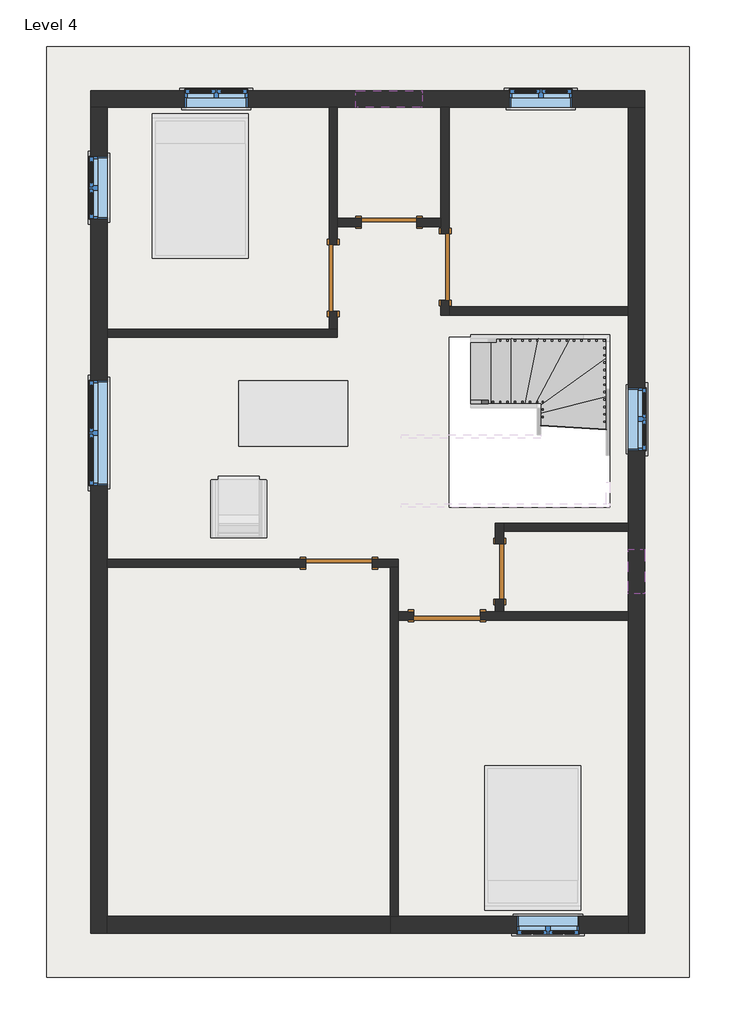
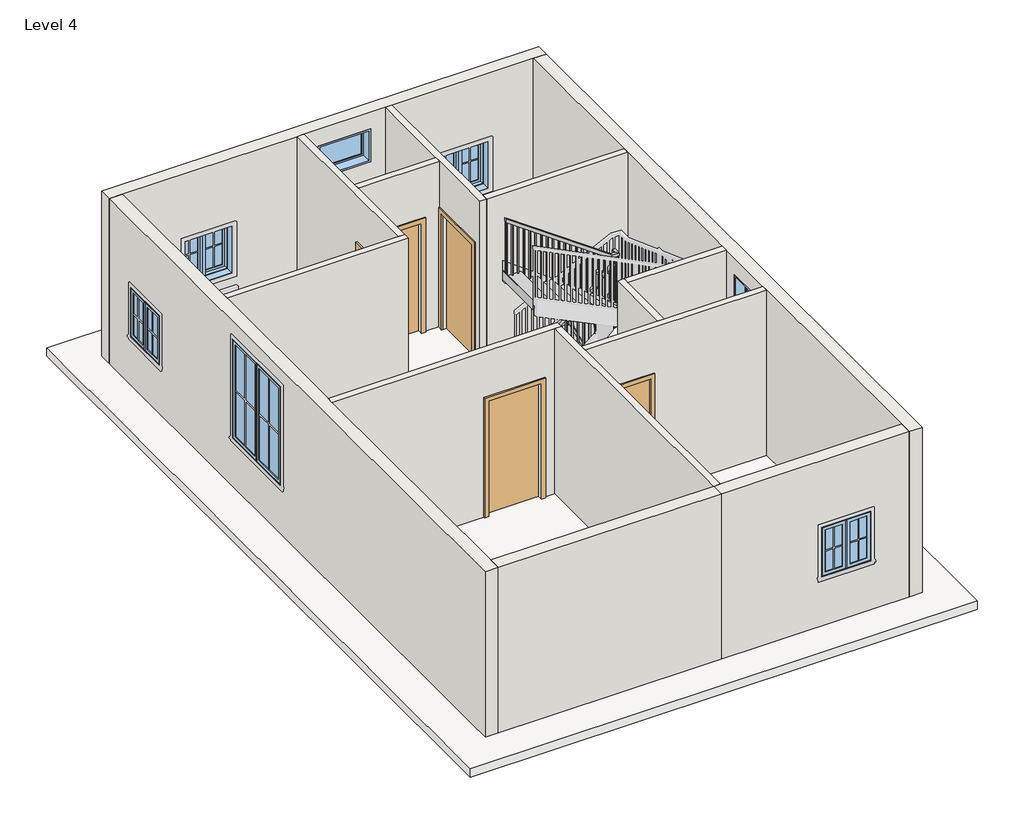
# One storey, part 1 of 2: 15 walls, 8 windows, 6 doors, 1 railing, 1 roof, 1 stair flight.
"""IFC4 building model written with IfcOpenShell, lengths in millimetres."""

from ifc_helpers import new_model, si_unit, frame, origin, place, context, project, spatial, polyline, outline, extrude, faceted_brep, transform, mapped, element, save
from components import door_d8f5dbb5, door_f2b275c1, door_e5f9f3c4, door_305aa2a5, stair_flight_52755f88, window_80340324, window_bb95b1c9, window_339605e1, window_9ac97e1a

model = new_model("IFC4")

# Units and contexts
model_context = context("Model", 3, world=origin())
ifc_project = project(units=[si_unit("LENGTHUNIT", "METRE", prefix="MILLI")], contexts=[model_context])

# Site, building, storey
site = spatial("IfcSite", under=ifc_project)
building = spatial("IfcBuilding", under=site)
storey = spatial("IfcBuildingStorey", under=building, Name="Level 4", Elevation=6400.8)

# Doors
placement = place(None, origin())
door_shape = door_d8f5dbb5(model_context)
element("IfcDoor", 1, ObjectType="Single-Flush : 30\" x 80\"", at=placement, inside=storey, context=model_context, shape_type="MappedRepresentation", body=[
    mapped(door_shape, transform((-963.1415084, 4519.6435985, 6400.8), x_axis=(1.0, 0.0, 0.0), y_axis=(0.0, 1.0, 0.0), z_axis=(0.0, 0.0, 1.0))),
])
door_2_shape = door_f2b275c1(model_context)
element("IfcDoor", 2, ObjectType="Single-Flush : 30\" x 80\"", at=placement, inside=storey, context=model_context, shape_type="MappedRepresentation", body=[
    mapped(door_2_shape, transform((554.5084916, -280.9564015, 6400.8), x_axis=(0.0, 1.0, 0.0), y_axis=(-1.0, 0.0, 0.0), z_axis=(0.0, 0.0, 1.0))),
])
door_3_shape = door_e5f9f3c4(model_context)
element("IfcDoor", 3, ObjectType="Single-Flush : 36\" x 84\"", at=placement, inside=storey, context=model_context, shape_type="MappedRepresentation", body=[
    mapped(door_3_shape, transform((-194.7915084, 3910.0435985, 6400.8), x_axis=(0.0, -1.0, 0.0), y_axis=(1.0, 0.0, 0.0), z_axis=(0.0, 0.0, 1.0))),
])
element("IfcDoor", 4, ObjectType="Single-Flush : 36\" x 84\"", at=placement, inside=storey, context=model_context, shape_type="MappedRepresentation", body=[
    mapped(door_3_shape, transform((-1655.2915084, -166.6564015, 6400.8), x_axis=(1.0, 0.0, 0.0), y_axis=(0.0, 1.0, 0.0), z_axis=(0.0, 0.0, 1.0))),
])
element("IfcDoor", 5, ObjectType="Single-Flush : 36\" x 84\"", at=placement, inside=storey, context=model_context, shape_type="MappedRepresentation", body=[
    mapped(door_3_shape, transform((-169.3915084, -890.5564015, 6400.8), x_axis=(-1.0, 0.0, 0.0), y_axis=(0.0, -1.0, 0.0), z_axis=(0.0, 0.0, 1.0))),
])
door_4_shape = door_305aa2a5(model_context)
element("IfcDoor", 6, ObjectType="Single-Flush : 36\" x 84\"", at=placement, inside=storey, context=model_context, shape_type="MappedRepresentation", body=[
    mapped(door_4_shape, transform((-1731.4915084, 3757.6435985, 6400.8), x_axis=(0.0, -1.0, 0.0), y_axis=(1.0, 0.0, 0.0), z_axis=(0.0, 0.0, 1.0))),
])

# Railing
element("IfcRailing", 7, ObjectType="Handrail - Rectangular", at=placement, inside=storey, context=model_context, shape_type="SolidModel", body=[
    faceted_brep([(158.6923968, 2074.8935985, 7484.5333333), (158.6923968, 2074.8935985, 7420.8053174), (158.6923968, 2024.0935985, 7420.8053174), (158.6923968, 2024.0935985, 7484.5333333), (1047.1901835, 2074.8935985, 8157.532376), (1097.9901835, 2074.8935985, 8132.2831856), (1097.9901835, 2024.0935985, 8132.2831856), (1047.1901835, 2024.0935985, 8157.532376), (1047.1901835, 2074.8935985, 8411.8303182), (1097.9901835, 2074.8935985, 8361.0303182), (1097.9901835, 2024.0935985, 8361.0303182), (1047.1901835, 2024.0935985, 8411.8303182), (1174.1901835, 2074.8935985, 8411.8303182), (1174.1901835, 2074.8935985, 8361.0303182), (1123.3901835, 2024.0935985, 8361.0303182), (1123.3901835, 2024.0935985, 8411.8303182), (1174.1901835, 1947.8935985, 8411.8303182), (1174.1901835, 1922.7437783, 8361.0303182), (1123.3901835, 1922.7437783, 8361.0303182), (1123.3901835, 1947.8935985, 8411.8303182), (1174.1901835, 1627.4476133, 8832.13697), (1174.1901835, 1576.6476133, 8814.9805221), (1123.3901835, 1576.6476133, 8814.9805221), (1123.3901835, 1627.4476133, 8832.13697), (1174.1901835, 1627.4476133, 9053.3821577), (1174.1901835, 1576.6476133, 9002.5821577), (1123.3901835, 1576.6476133, 9002.5821577), (1123.3901835, 1627.4476133, 9053.3821577), (1174.1901835, 1500.4476133, 9053.3821577), (1174.1901835, 1500.4476133, 9002.5821577), (1123.3901835, 1551.2476133, 9002.5821577), (1123.3901835, 1551.2476133, 9053.3821577), (1047.1901835, 1500.4476133, 9053.3821577), (1030.9951821, 1500.4476133, 9002.5821577), (1030.9951821, 1551.2476133, 9002.5821577), (1047.1901835, 1551.2476133, 9053.3821577), (-798.3242294, 1500.4476133, 10363.2), (-798.3242294, 1551.2476133, 10363.2), (-798.3242294, 1551.2476133, 10300.9059138), (-798.3242294, 1500.4476133, 10300.9059138)], [[[0, 1, 2, 3]], [[1, 0, 4, 5]], [[2, 1, 5, 6]], [[3, 2, 6, 7]], [[0, 3, 7, 4]], [[5, 4, 8, 9]], [[6, 5, 9, 10]], [[7, 6, 10, 11]], [[4, 7, 11, 8]], [[9, 8, 12, 13]], [[10, 9, 13, 14]], [[11, 10, 14, 15]], [[8, 11, 15, 12]], [[13, 12, 16, 17]], [[14, 13, 17, 18]], [[15, 14, 18, 19]], [[12, 15, 19, 16]], [[17, 16, 20, 21]], [[18, 17, 21, 22]], [[19, 18, 22, 23]], [[16, 19, 23, 20]], [[21, 20, 24, 25]], [[22, 21, 25, 26]], [[23, 22, 26, 27]], [[20, 23, 27, 24]], [[25, 24, 28, 29]], [[26, 25, 29, 30]], [[27, 26, 30, 31]], [[24, 27, 31, 28]], [[29, 28, 32, 33]], [[30, 29, 33, 34]], [[31, 30, 34, 35]], [[28, 31, 35, 32]], [[36, 37, 38, 39]], [[33, 32, 36, 39]], [[34, 33, 39, 38]], [[35, 34, 38, 37]], [[32, 35, 37, 36]]]),
    extrude(outline(polyline([(10282.2830025, -772.0848165), (10295.8033683, -791.1348165), (9279.4666667, -791.1348165), (9279.4666667, -772.0848165), (10282.2830025, -772.0848165)])), frame((0.0, 1516.3226133, 0.0), z_axis=(0.0, 1.0, 0.0), x_axis=(0.0, 0.0, 1.0)), (0.0, 0.0, 1.0), 19.05),
    extrude(outline(polyline([(10210.1743851, -670.4848165), (10223.6947509, -689.5348165), (9279.4666667, -689.5348165), (9279.4666667, -670.4848165), (10210.1743851, -670.4848165)])), frame((0.0, 1516.3226133, 0.0), z_axis=(0.0, 1.0, 0.0), x_axis=(0.0, 0.0, 1.0)), (0.0, 0.0, 1.0), 19.05),
    extrude(outline(polyline([(10138.0657677, -568.8848165), (10151.5861334, -587.9348165), (9279.4666667, -587.9348165), (9279.4666667, -568.8848165), (10138.0657677, -568.8848165)])), frame((0.0, 1516.3226133, 0.0), z_axis=(0.0, 1.0, 0.0), x_axis=(0.0, 0.0, 1.0)), (0.0, 0.0, 1.0), 19.05),
    extrude(outline(polyline([(10065.9571502, -467.2848165), (10079.477516, -486.3348165), (9110.1333333, -486.3348165), (9110.1333333, -467.2848165), (10065.9571502, -467.2848165)])), frame((0.0, 1516.3226133, 0.0), z_axis=(0.0, 1.0, 0.0), x_axis=(0.0, 0.0, 1.0)), (0.0, 0.0, 1.0), 19.05),
    extrude(outline(polyline([(9993.8485328, -365.6848165), (10007.3688986, -384.7348165), (9110.1333333, -384.7348165), (9110.1333333, -365.6848165), (9993.8485328, -365.6848165)])), frame((0.0, 1516.3226133, 0.0), z_axis=(0.0, 1.0, 0.0), x_axis=(0.0, 0.0, 1.0)), (0.0, 0.0, 1.0), 19.05),
    extrude(outline(polyline([(9921.7399154, -264.0848165), (9935.2602811, -283.1348165), (9110.1333333, -283.1348165), (9110.1333333, -264.0848165), (9921.7399154, -264.0848165)])), frame((0.0, 1516.3226133, 0.0), z_axis=(0.0, 1.0, 0.0), x_axis=(0.0, 0.0, 1.0)), (0.0, 0.0, 1.0), 19.05),
    extrude(outline(polyline([(9849.6312979, -162.4848165), (9863.1516637, -181.5348165), (8940.8, -181.5348165), (8940.8, -162.4848165), (9849.6312979, -162.4848165)])), frame((0.0, 1516.3226133, 0.0), z_axis=(0.0, 1.0, 0.0), x_axis=(0.0, 0.0, 1.0)), (0.0, 0.0, 1.0), 19.05),
    extrude(outline(polyline([(9777.5226805, -60.8848165), (9791.0430462, -79.9348165), (8940.8, -79.9348165), (8940.8, -60.8848165), (9777.5226805, -60.8848165)])), frame((0.0, 1516.3226133, 0.0), z_axis=(0.0, 1.0, 0.0), x_axis=(0.0, 0.0, 1.0)), (0.0, 0.0, 1.0), 19.05),
    extrude(outline(polyline([(9705.414063, 40.7151835), (9718.9344288, 21.6651835), (8771.4666667, 21.6651835), (8771.4666667, 40.7151835), (9705.414063, 40.7151835)])), frame((0.0, 1516.3226133, 0.0), z_axis=(0.0, 1.0, 0.0), x_axis=(0.0, 0.0, 1.0)), (0.0, 0.0, 1.0), 19.05),
    extrude(outline(polyline([(9633.3054456, 142.3151835), (9646.8258114, 123.2651835), (8771.4666667, 123.2651835), (8771.4666667, 142.3151835), (9633.3054456, 142.3151835)])), frame((0.0, 1516.3226133, 0.0), z_axis=(0.0, 1.0, 0.0), x_axis=(0.0, 0.0, 1.0)), (0.0, 0.0, 1.0), 19.05),
    extrude(outline(polyline([(9561.1968282, 243.9151835), (9574.7171939, 224.8651835), (8771.4666667, 224.8651835), (8771.4666667, 243.9151835), (9561.1968282, 243.9151835)])), frame((0.0, 1516.3226133, 0.0), z_axis=(0.0, 1.0, 0.0), x_axis=(0.0, 0.0, 1.0)), (0.0, 0.0, 1.0), 19.05),
    extrude(outline(polyline([(9489.0882107, 345.5151835), (9502.6085765, 326.4651835), (8602.1333333, 326.4651835), (8602.1333333, 345.5151835), (9489.0882107, 345.5151835)])), frame((0.0, 1516.3226133, 0.0), z_axis=(0.0, 1.0, 0.0), x_axis=(0.0, 0.0, 1.0)), (0.0, 0.0, 1.0), 19.05),
    extrude(outline(polyline([(9416.9795933, 447.1151835), (9430.4999591, 428.0651835), (8602.1333333, 428.0651835), (8602.1333333, 447.1151835), (9416.9795933, 447.1151835)])), frame((0.0, 1516.3226133, 0.0), z_axis=(0.0, 1.0, 0.0), x_axis=(0.0, 0.0, 1.0)), (0.0, 0.0, 1.0), 19.05),
    extrude(outline(polyline([(9344.8709758, 548.7151835), (9358.3913416, 529.6651835), (8432.8, 529.6651835), (8432.8, 548.7151835), (9344.8709758, 548.7151835)])), frame((0.0, 1516.3226133, 0.0), z_axis=(0.0, 1.0, 0.0), x_axis=(0.0, 0.0, 1.0)), (0.0, 0.0, 1.0), 19.05),
    extrude(outline(polyline([(9272.7623584, 650.3151835), (9286.2827242, 631.2651835), (8432.8, 631.2651835), (8432.8, 650.3151835), (9272.7623584, 650.3151835)])), frame((0.0, 1516.3226133, 0.0), z_axis=(0.0, 1.0, 0.0), x_axis=(0.0, 0.0, 1.0)), (0.0, 0.0, 1.0), 19.05),
    extrude(outline(polyline([(9200.653741, 751.9151835), (9214.1741067, 732.8651835), (8432.8, 732.8651835), (8432.8, 751.9151835), (9200.653741, 751.9151835)])), frame((0.0, 1516.3226133, 0.0), z_axis=(0.0, 1.0, 0.0), x_axis=(0.0, 0.0, 1.0)), (0.0, 0.0, 1.0), 19.05),
    extrude(outline(polyline([(9128.5451235, 853.5151835), (9142.0654893, 834.4651835), (8263.4666667, 834.4651835), (8263.4666667, 853.5151835), (9128.5451235, 853.5151835)])), frame((0.0, 1516.3226133, 0.0), z_axis=(0.0, 1.0, 0.0), x_axis=(0.0, 0.0, 1.0)), (0.0, 0.0, 1.0), 19.05),
    extrude(outline(polyline([(9056.4365061, 955.1151835), (9069.9568719, 936.0651835), (8263.4666667, 936.0651835), (8263.4666667, 955.1151835), (9056.4365061, 955.1151835)])), frame((0.0, 1516.3226133, 0.0), z_axis=(0.0, 1.0, 0.0), x_axis=(0.0, 0.0, 1.0)), (0.0, 0.0, 1.0), 19.05),
    extrude(outline(polyline([(8984.3278887, 1056.7151835), (8997.8482544, 1037.6651835), (8094.1333333, 1037.6651835), (8094.1333333, 1056.7151835), (8984.3278887, 1056.7151835)])), frame((0.0, 1516.3226133, 0.0), z_axis=(0.0, 1.0, 0.0), x_axis=(0.0, 0.0, 1.0)), (0.0, 0.0, 1.0), 19.05),
    extrude(outline(polyline([(1139.2651835, 1551.0185985), (1158.3151835, 1551.0185985), (1158.3151835, 1531.9685985), (1139.2651835, 1531.9685985), (1139.2651835, 1551.0185985)])), frame((0.0, 0.0, 7924.8), z_axis=(0.0, 0.0, 1.0), x_axis=(1.0, 0.0, 0.0)), (0.0, 0.0, 1.0), 1077.7821578),
    extrude(outline(polyline([(1633.5685985, 8740.3212353), (1652.6185985, 8715.3346787), (1652.6185985, 7755.4666667), (1633.5685985, 7755.4666667), (1633.5685985, 8740.3212353)])), frame((1139.2651835, 0.0, 0.0), z_axis=(1.0, 0.0, 0.0), x_axis=(0.0, 1.0, 0.0)), (0.0, 0.0, 1.0), 19.05),
    extrude(outline(polyline([(1735.1685985, 8607.0596006), (1754.2185985, 8582.073044), (1754.2185985, 7755.4666667), (1735.1685985, 7755.4666667), (1735.1685985, 8607.0596006)])), frame((1139.2651835, 0.0, 0.0), z_axis=(1.0, 0.0, 0.0), x_axis=(0.0, 1.0, 0.0)), (0.0, 0.0, 1.0), 19.05),
    extrude(outline(polyline([(1836.7685985, 8473.7979659), (1855.8185985, 8448.8114093), (1855.8185985, 7586.1333333), (1836.7685985, 7586.1333333), (1836.7685985, 8473.7979659)])), frame((1139.2651835, 0.0, 0.0), z_axis=(1.0, 0.0, 0.0), x_axis=(0.0, 1.0, 0.0)), (0.0, 0.0, 1.0), 19.05),
    extrude(outline(polyline([(1938.3685985, 8340.5363312), (1957.4185985, 8315.5497746), (1957.4185985, 7416.8), (1938.3685985, 7416.8), (1938.3685985, 8340.5363312)])), frame((1139.2651835, 0.0, 0.0), z_axis=(1.0, 0.0, 0.0), x_axis=(0.0, 1.0, 0.0)), (0.0, 0.0, 1.0), 19.05),
    extrude(outline(polyline([(1063.5673968, 2039.9685985), (1063.5673968, 2059.0185985), (1082.6173968, 2059.0185985), (1082.6173968, 2039.9685985), (1063.5673968, 2039.9685985)])), frame((0.0, 0.0, 7247.4666667), z_axis=(0.0, 0.0, 1.0), x_axis=(1.0, 0.0, 0.0)), (0.0, 0.0, 1.0), 1113.5636515),
    extrude(outline(polyline([(8043.6813066, 981.0173968), (8029.251747, 961.9673968), (7078.1333333, 961.9673968), (7078.1333333, 981.0173968), (8043.6813066, 981.0173968)])), frame((0.0, 2039.9685985, 0.0), z_axis=(0.0, 1.0, 0.0), x_axis=(0.0, 0.0, 1.0)), (0.0, 0.0, 1.0), 19.05),
    extrude(outline(polyline([(7966.7236554, 879.4173968), (7952.2940958, 860.3673968), (6908.8, 860.3673968), (6908.8, 879.4173968), (7966.7236554, 879.4173968)])), frame((0.0, 2039.9685985, 0.0), z_axis=(0.0, 1.0, 0.0), x_axis=(0.0, 0.0, 1.0)), (0.0, 0.0, 1.0), 19.05),
    extrude(outline(polyline([(7889.7660042, 777.8173968), (7875.3364446, 758.7673968), (6908.8, 758.7673968), (6908.8, 777.8173968), (7889.7660042, 777.8173968)])), frame((0.0, 2039.9685985, 0.0), z_axis=(0.0, 1.0, 0.0), x_axis=(0.0, 0.0, 1.0)), (0.0, 0.0, 1.0), 19.05),
    extrude(outline(polyline([(7812.808353, 676.2173968), (7798.3787934, 657.1673968), (6739.4666667, 657.1673968), (6739.4666667, 676.2173968), (7812.808353, 676.2173968)])), frame((0.0, 2039.9685985, 0.0), z_axis=(0.0, 1.0, 0.0), x_axis=(0.0, 0.0, 1.0)), (0.0, 0.0, 1.0), 19.05),
    extrude(outline(polyline([(7735.8507019, 574.6173968), (7721.4211423, 555.5673968), (6739.4666667, 555.5673968), (6739.4666667, 574.6173968), (7735.8507019, 574.6173968)])), frame((0.0, 2039.9685985, 0.0), z_axis=(0.0, 1.0, 0.0), x_axis=(0.0, 0.0, 1.0)), (0.0, 0.0, 1.0), 19.05),
    extrude(outline(polyline([(7658.8930507, 473.0173968), (7644.4634911, 453.9673968), (6739.4666667, 453.9673968), (6739.4666667, 473.0173968), (7658.8930507, 473.0173968)])), frame((0.0, 2039.9685985, 0.0), z_axis=(0.0, 1.0, 0.0), x_axis=(0.0, 0.0, 1.0)), (0.0, 0.0, 1.0), 19.05),
    extrude(outline(polyline([(7581.9353995, 371.4173968), (7567.5058399, 352.3673968), (6570.1333333, 352.3673968), (6570.1333333, 371.4173968), (7581.9353995, 371.4173968)])), frame((0.0, 2039.9685985, 0.0), z_axis=(0.0, 1.0, 0.0), x_axis=(0.0, 0.0, 1.0)), (0.0, 0.0, 1.0), 19.05),
    extrude(outline(polyline([(7504.9777483, 269.8173968), (7490.5481887, 250.7673968), (6570.1333333, 250.7673968), (6570.1333333, 269.8173968), (7504.9777483, 269.8173968)])), frame((0.0, 2039.9685985, 0.0), z_axis=(0.0, 1.0, 0.0), x_axis=(0.0, 0.0, 1.0)), (0.0, 0.0, 1.0), 19.05),
    extrude(outline(polyline([(1139.2651835, 1535.3726133), (1158.3151835, 1535.3726133), (1158.3151835, 1516.3226133), (1139.2651835, 1516.3226133), (1139.2651835, 1535.3726133)])), frame((0.0, 0.0, 7924.8), z_axis=(0.0, 0.0, 1.0), x_axis=(1.0, 0.0, 0.0)), (0.0, 0.0, 1.0), 1077.7821578),
    extrude(outline(polyline([(1139.2651835, 2039.9685985), (1139.2651835, 2059.0185985), (1158.3151835, 2059.0185985), (1158.3151835, 2039.9685985), (1139.2651835, 2039.9685985)])), frame((0.0, 0.0, 7247.4666667), z_axis=(0.0, 0.0, 1.0), x_axis=(1.0, 0.0, 0.0)), (0.0, 0.0, 1.0), 1113.5636515),
    extrude(outline(polyline([(10287.385548, -779.2742294), (10300.9059138, -798.3242294), (9279.4666667, -798.3242294), (9279.4666667, -779.2742294), (10287.385548, -779.2742294)])), frame((0.0, 1516.3226133, 0.0), z_axis=(0.0, 1.0, 0.0), x_axis=(0.0, 0.0, 1.0)), (0.0, 0.0, 1.0), 19.05),
    extrude(outline(polyline([(7435.234877, 177.7423968), (7420.8053174, 158.6923968), (6570.1333333, 158.6923968), (6570.1333333, 177.7423968), (7435.234877, 177.7423968)])), frame((0.0, 2039.9685985, 0.0), z_axis=(0.0, 1.0, 0.0), x_axis=(0.0, 0.0, 1.0)), (0.0, 0.0, 1.0), 19.05),
])

# Roof
element("IfcRoof", 8, ObjectType="Generic - 12\"", at=placement, inside=storey, context=model_context, shape_type="SweptSolid", body=[
    extrude(outline(polyline([(3164.3584916, 6938.9935985), (3164.3584916, -5862.6064015), (-5674.8415084, -5862.6064015), (-5674.8415084, 6938.9935985), (3164.3584916, 6938.9935985)]), holes=[polyline([(2072.9441983, 2938.4935985), (-137.6415084, 2938.4935985), (-137.6415084, 601.6935985), (2072.9441983, 601.6935985), (2072.9441983, 2938.4935985)])]), frame((0.0, 0.0, 6248.4), z_axis=(0.0, 0.0, 1.0), x_axis=(1.0, 0.0, 0.0)), (0.0, 0.0, 1.0), 152.4),
])

# Stair flight
stair_flight_shape = stair_flight_52755f88(model_context)
element("IfcStairFlight", 9, ObjectType="2\" Tread 1\" Nosing 1/4\" Riser", at=placement, inside=storey, context=model_context, shape_type="MappedRepresentation", body=[
    mapped(stair_flight_shape, transform((0.0, 0.0, 0.0), x_axis=(1.0, 0.0, 0.0), y_axis=(0.0, 1.0, 0.0), z_axis=(0.0, 0.0, 1.0))),
])

# Walls
element("IfcWall", 10, ObjectType="WALL4.5\"", at=placement, inside=storey, context=model_context, shape_type="Brep", body=[
    faceted_brep([(-4836.6415084, 2938.4935985, 6400.8), (-1674.3415084, 2938.4935985, 6400.8), (-1674.3415084, 2938.4935985, 9448.8), (-4836.6415084, 2938.4935985, 9448.8), (-4836.6415084, 3052.7935985, 6400.8), (-4836.6415084, 3052.7935985, 9448.8), (-1788.6415084, 3052.7935985, 9448.8), (-1674.3415084, 3052.7935985, 9448.8), (-1674.3415084, 3052.7935985, 6400.8), (-1788.6415084, 3052.7935985, 6400.8)], [[[0, 1, 2, 3]], [[4, 5, 6, 7, 8, 9]], [[1, 0, 4, 9, 8]], [[0, 3, 5, 4]], [[2, 1, 8, 7]], [[3, 2, 7, 6, 5]]]),
])
element("IfcWall", 11, ObjectType="WALL4.5\"", at=placement, inside=storey, context=model_context, shape_type="Brep", body=[
    faceted_brep([(-1674.3415084, 3052.7935985, 6400.8), (-1674.3415084, 3300.4435985, 6400.8), (-1674.3415084, 3300.4435985, 8534.4), (-1674.3415084, 4214.8435985, 8534.4), (-1674.3415084, 4214.8435985, 6400.8), (-1674.3415084, 4462.4935985, 6400.8), (-1674.3415084, 4576.7935985, 6400.8), (-1674.3415084, 6100.7935985, 6400.8), (-1674.3415084, 6100.7935985, 9448.8), (-1674.3415084, 4576.7935985, 9448.8), (-1674.3415084, 4462.4935985, 9448.8), (-1674.3415084, 3052.7935985, 9448.8), (-1788.6415084, 3300.4435985, 8534.4), (-1788.6415084, 3300.4435985, 6400.8), (-1788.6415084, 3052.7935985, 6400.8), (-1788.6415084, 3052.7935985, 9448.8), (-1788.6415084, 6100.7935985, 9448.8), (-1788.6415084, 6100.7935985, 6400.8), (-1788.6415084, 4214.8435985, 6400.8), (-1788.6415084, 4214.8435985, 8534.4)], [[[0, 1, 2, 3, 4, 5, 6, 7, 8, 9, 10, 11]], [[12, 13, 14, 15, 16, 17, 18, 19]], [[18, 17, 7, 6, 5, 4]], [[14, 13, 1, 0]], [[0, 11, 15, 14]], [[8, 7, 17, 16]], [[2, 1, 13, 12]], [[3, 2, 12, 19]], [[4, 3, 19, 18]], [[11, 10, 9, 8, 16, 15]]]),
])
element("IfcWall", 12, ObjectType="WALL4.5\"", at=placement, inside=storey, context=model_context, shape_type="SweptSolid", body=[
    extrude(outline(polyline([(8432.8, -582.1415084), (6400.8, -582.1415084), (6400.8, -251.9415084), (9448.8, -251.9415084), (9448.8, -1674.3415084), (6400.8, -1674.3415084), (6400.8, -1344.1415084), (8432.8, -1344.1415084), (8432.8, -582.1415084)])), frame((0.0, 4462.4935985, 0.0), z_axis=(0.0, 1.0, 0.0), x_axis=(0.0, 0.0, 1.0)), (0.0, 0.0, 1.0), 114.3),
])
element("IfcWall", 13, ObjectType="WALL4.5\"", at=placement, inside=storey, context=model_context, shape_type="Brep", body=[
    faceted_brep([(-251.9415084, 3452.8435985, 8534.4), (-251.9415084, 3452.8435985, 6400.8), (-251.9415084, 3243.2935985, 6400.8), (-251.9415084, 3243.2935985, 9448.8), (-251.9415084, 4462.4935985, 9448.8), (-251.9415084, 4576.7935985, 9448.8), (-251.9415084, 6100.7935985, 9448.8), (-251.9415084, 6100.7935985, 6400.8), (-251.9415084, 4576.7935985, 6400.8), (-251.9415084, 4462.4935985, 6400.8), (-251.9415084, 4367.2435985, 6400.8), (-251.9415084, 4367.2435985, 8534.4), (-137.6415084, 3243.2935985, 6400.8), (-137.6415084, 3357.5935985, 6400.8), (-137.6415084, 3452.8435985, 6400.8), (-137.6415084, 3452.8435985, 8534.4), (-137.6415084, 4367.2435985, 8534.4), (-137.6415084, 4367.2435985, 6400.8), (-137.6415084, 6100.7935985, 6400.8), (-137.6415084, 6100.7935985, 9448.8), (-137.6415084, 3357.5935985, 9448.8), (-137.6415084, 3243.2935985, 9448.8)], [[[0, 1, 2, 3, 4, 5, 6, 7, 8, 9, 10, 11]], [[12, 13, 14, 15, 16, 17, 18, 19, 20, 21]], [[2, 1, 14, 13, 12]], [[10, 9, 8, 7, 18, 17]], [[7, 6, 19, 18]], [[3, 2, 12, 21]], [[15, 14, 1, 0]], [[16, 15, 0, 11]], [[17, 16, 11, 10]], [[6, 5, 4, 3, 21, 20, 19]]]),
])
element("IfcWall", 14, ObjectType="WALL4.5\"", at=placement, inside=storey, context=model_context, shape_type="SweptSolid", body=[
    extrude(outline(polyline([(2326.1584916, 3243.2935985), (-137.6415084, 3243.2935985), (-137.6415084, 3357.5935985), (2326.1584916, 3357.5935985), (2326.1584916, 3243.2935985)])), frame((0.0, 0.0, 6400.8), z_axis=(0.0, 0.0, 1.0), x_axis=(1.0, 0.0, 0.0)), (0.0, 0.0, 1.0), 3048.0),
])
element("IfcWall", 15, ObjectType="WALL4.5\"", at=placement, inside=storey, context=model_context, shape_type="Brep", body=[
    faceted_brep([(-1198.0915084, -223.8064015, 8534.4), (-1198.0915084, -223.8064015, 6400.8), (-950.4415084, -223.8064015, 6400.8), (-836.1415084, -223.8064015, 6400.8), (-836.1415084, -223.8064015, 9448.8), (-950.4415084, -223.8064015, 9448.8), (-4836.6415084, -223.8064015, 9448.8), (-4836.6415084, -223.8064015, 6400.8), (-2112.4915084, -223.8064015, 6400.8), (-2112.4915084, -223.8064015, 8534.4), (-836.1415084, -109.5064015, 6400.8), (-1198.0915084, -109.5064015, 6400.8), (-1198.0915084, -109.5064015, 8534.4), (-2112.4915084, -109.5064015, 8534.4), (-2112.4915084, -109.5064015, 6400.8), (-4836.6415084, -109.5064015, 6400.8), (-4836.6415084, -109.5064015, 9448.8), (-836.1415084, -109.5064015, 9448.8)], [[[0, 1, 2, 3, 4, 5, 6, 7, 8, 9]], [[10, 11, 12, 13, 14, 15, 16, 17]], [[8, 7, 15, 14]], [[3, 2, 1, 11, 10]], [[7, 6, 16, 15]], [[4, 3, 10, 17]], [[12, 11, 1, 0]], [[13, 12, 0, 9]], [[14, 13, 9, 8]], [[6, 5, 4, 17, 16]]]),
])
element("IfcWall", 16, ObjectType="WALL4.5\"", at=placement, inside=storey, context=model_context, shape_type="Brep", body=[
    faceted_brep([(-950.4415084, -223.8064015, 6400.8), (-950.4415084, -5024.4064015, 6400.8), (-950.4415084, -5024.4064015, 9448.8), (-950.4415084, -223.8064015, 9448.8), (-836.1415084, -223.8064015, 6400.8), (-836.1415084, -223.8064015, 9448.8), (-836.1415084, -833.4064015, 9448.8), (-836.1415084, -947.7064015, 9448.8), (-836.1415084, -5024.4064015, 9448.8), (-836.1415084, -5024.4064015, 6400.8), (-836.1415084, -947.7064015, 6400.8), (-836.1415084, -833.4064015, 6400.8)], [[[0, 1, 2, 3]], [[4, 5, 6, 7, 8, 9, 10, 11]], [[2, 1, 9, 8]], [[0, 3, 5, 4]], [[1, 0, 4, 11, 10, 9]], [[3, 2, 8, 7, 6, 5]]]),
])
element("IfcWall", 17, ObjectType="WALL4.5\"", at=placement, inside=storey, context=model_context, shape_type="Brep", body=[
    faceted_brep([(-836.1415084, -947.7064015, 6400.8), (-626.5915084, -947.7064015, 6400.8), (-626.5915084, -947.7064015, 8534.4), (287.8084916, -947.7064015, 8534.4), (287.8084916, -947.7064015, 6400.8), (2326.1584916, -947.7064015, 6400.8), (2326.1584916, -947.7064015, 9448.8), (-836.1415084, -947.7064015, 9448.8), (-626.5915084, -833.4064015, 8534.4), (-626.5915084, -833.4064015, 6400.8), (-836.1415084, -833.4064015, 6400.8), (-836.1415084, -833.4064015, 9448.8), (497.3584916, -833.4064015, 9448.8), (611.6584916, -833.4064015, 9448.8), (2326.1584916, -833.4064015, 9448.8), (2326.1584916, -833.4064015, 6400.8), (611.6584916, -833.4064015, 6400.8), (497.3584916, -833.4064015, 6400.8), (287.8084916, -833.4064015, 6400.8), (287.8084916, -833.4064015, 8534.4)], [[[0, 1, 2, 3, 4, 5, 6, 7]], [[8, 9, 10, 11, 12, 13, 14, 15, 16, 17, 18, 19]], [[10, 9, 1, 0]], [[18, 17, 16, 15, 5, 4]], [[6, 5, 15, 14]], [[0, 7, 11, 10]], [[2, 1, 9, 8]], [[3, 2, 8, 19]], [[4, 3, 19, 18]], [[7, 6, 14, 13, 12, 11]]]),
])
element("IfcWall", 18, ObjectType="WALL4.5\"", at=placement, inside=storey, context=model_context, shape_type="Brep", body=[
    faceted_brep([(611.6584916, 100.0435985, 8432.8), (611.6584916, 100.0435985, 6400.8), (611.6584916, 271.4935985, 6400.8), (611.6584916, 385.7935985, 6400.8), (611.6584916, 385.7935985, 9448.8), (611.6584916, 271.4935985, 9448.8), (611.6584916, -833.4064015, 9448.8), (611.6584916, -833.4064015, 6400.8), (611.6584916, -661.9564015, 6400.8), (611.6584916, -661.9564015, 8432.8), (497.3584916, 385.7935985, 6400.8), (497.3584916, 100.0435985, 6400.8), (497.3584916, 100.0435985, 8432.8), (497.3584916, -661.9564015, 8432.8), (497.3584916, -661.9564015, 6400.8), (497.3584916, -833.4064015, 6400.8), (497.3584916, -833.4064015, 9448.8), (497.3584916, 385.7935985, 9448.8)], [[[0, 1, 2, 3, 4, 5, 6, 7, 8, 9]], [[10, 11, 12, 13, 14, 15, 16, 17]], [[8, 7, 15, 14]], [[3, 2, 1, 11, 10]], [[7, 6, 16, 15]], [[4, 3, 10, 17]], [[12, 11, 1, 0]], [[13, 12, 0, 9]], [[14, 13, 9, 8]], [[6, 5, 4, 17, 16]]]),
])
element("IfcWall", 19, ObjectType="WALL4.5\"", at=placement, inside=storey, context=model_context, shape_type="SweptSolid", body=[
    extrude(outline(polyline([(2326.1584916, 271.4935985), (611.6584916, 271.4935985), (611.6584916, 385.7935985), (2326.1584916, 385.7935985), (2326.1584916, 271.4935985)])), frame((0.0, 0.0, 6400.8), z_axis=(0.0, 0.0, 1.0), x_axis=(1.0, 0.0, 0.0)), (0.0, 0.0, 1.0), 3048.0),
])
element("IfcWall", 20, ObjectType="WALL9\"", at=placement, inside=storey, context=model_context, shape_type="Brep", body=[
    faceted_brep([(-5065.2415084, 6100.7935985, 6400.8), (-4836.6415084, 6100.7935985, 6400.8), (-1788.6415084, 6100.7935985, 6400.8), (-1674.3415084, 6100.7935985, 6400.8), (-251.9415084, 6100.7935985, 6400.8), (-137.6415084, 6100.7935985, 6400.8), (2326.1584916, 6100.7935985, 6400.8), (2554.7584916, 6100.7935985, 6400.8), (2554.7584916, 6100.7935985, 9448.8), (2326.1584916, 6100.7935985, 9448.8), (-137.6415084, 6100.7935985, 9448.8), (-251.9415084, 6100.7935985, 9448.8), (-1674.3415084, 6100.7935985, 9448.8), (-1788.6415084, 6100.7935985, 9448.8), (-4836.6415084, 6100.7935985, 9448.8), (-5065.2415084, 6100.7935985, 9448.8), (-505.9415084, 6100.7935985, 9144.0), (-505.9415084, 6100.7935985, 8534.4), (-1420.3415084, 6100.7935985, 8534.4), (-1420.3415084, 6100.7935985, 9144.0), (-2909.4165084, 6100.7935985, 8229.6), (-2909.4165084, 6100.7935985, 7315.2), (-3773.0165084, 6100.7935985, 7315.2), (-3773.0165084, 6100.7935985, 8229.6), (1554.6334916, 6100.7935985, 8229.6), (1554.6334916, 6100.7935985, 7315.2), (691.0334916, 6100.7935985, 7315.2), (691.0334916, 6100.7935985, 8229.6), (-5065.2415084, 6329.3935985, 6400.8), (-5065.2415084, 6329.3935985, 9448.8), (2554.7584916, 6329.3935985, 9448.8), (2554.7584916, 6329.3935985, 6400.8), (-505.9415084, 6329.3935985, 9144.0), (-1420.3415084, 6329.3935985, 9144.0), (-1420.3415084, 6329.3935985, 8534.4), (-505.9415084, 6329.3935985, 8534.4), (-2909.4165084, 6329.3935985, 8229.6), (-3773.0165084, 6329.3935985, 8229.6), (-3773.0165084, 6329.3935985, 7315.2), (-2909.4165084, 6329.3935985, 7315.2), (1554.6334916, 6329.3935985, 8229.6), (691.0334916, 6329.3935985, 8229.6), (691.0334916, 6329.3935985, 7315.2), (1554.6334916, 6329.3935985, 7315.2)], [[[0, 1, 2, 3, 4, 5, 6, 7, 8, 9, 10, 11, 12, 13, 14, 15], [16, 17, 18, 19], [20, 21, 22, 23], [24, 25, 26, 27]], [[28, 29, 30, 31], [32, 33, 34, 35], [36, 37, 38, 39], [40, 41, 42, 43]], [[7, 6, 5, 4, 3, 2, 1, 0, 28, 31]], [[8, 7, 31, 30]], [[0, 15, 29, 28]], [[17, 16, 32, 35]], [[18, 17, 35, 34]], [[19, 18, 34, 33]], [[16, 19, 33, 32]], [[21, 20, 36, 39]], [[22, 21, 39, 38]], [[23, 22, 38, 37]], [[20, 23, 37, 36]], [[25, 24, 40, 43]], [[26, 25, 43, 42]], [[27, 26, 42, 41]], [[24, 27, 41, 40]], [[15, 14, 13, 12, 11, 10, 9, 8, 30, 29]]]),
])
element("IfcWall", 21, ObjectType="WALL9\"", at=placement, inside=storey, context=model_context, shape_type="Brep", body=[
    faceted_brep([(2326.1584916, 6100.7935985, 6400.8), (2326.1584916, 3357.5935985, 6400.8), (2326.1584916, 3243.2935985, 6400.8), (2326.1584916, 385.7935985, 6400.8), (2326.1584916, 271.4935985, 6400.8), (2326.1584916, -833.4064015, 6400.8), (2326.1584916, -947.7064015, 6400.8), (2326.1584916, -5024.4064015, 6400.8), (2326.1584916, -5253.0064015, 6400.8), (2326.1584916, -5253.0064015, 9448.8), (2326.1584916, -5024.4064015, 9448.8), (2326.1584916, -947.7064015, 9448.8), (2326.1584916, -833.4064015, 9448.8), (2326.1584916, 271.4935985, 9448.8), (2326.1584916, 385.7935985, 9448.8), (2326.1584916, 3243.2935985, 9448.8), (2326.1584916, 3357.5935985, 9448.8), (2326.1584916, 6100.7935985, 9448.8), (2326.1584916, -585.7564015, 9144.0), (2326.1584916, -585.7564015, 8534.4), (2326.1584916, 23.8435985, 8534.4), (2326.1584916, 23.8435985, 9144.0), (2326.1584916, 1382.7435985, 8229.6), (2326.1584916, 1382.7435985, 7315.2), (2326.1584916, 2246.3435985, 7315.2), (2326.1584916, 2246.3435985, 8229.6), (2554.7584916, 6100.7935985, 6400.8), (2554.7584916, 6100.7935985, 9448.8), (2554.7584916, -5253.0064015, 9448.8), (2554.7584916, -5253.0064015, 6400.8), (2554.7584916, -585.7564015, 9144.0), (2554.7584916, 23.8435985, 9144.0), (2554.7584916, 23.8435985, 8534.4), (2554.7584916, -585.7564015, 8534.4), (2554.7584916, 1382.7435985, 8229.6), (2554.7584916, 2246.3435985, 8229.6), (2554.7584916, 2246.3435985, 7315.2), (2554.7584916, 1382.7435985, 7315.2)], [[[0, 1, 2, 3, 4, 5, 6, 7, 8, 9, 10, 11, 12, 13, 14, 15, 16, 17], [18, 19, 20, 21], [22, 23, 24, 25]], [[26, 27, 28, 29], [30, 31, 32, 33], [34, 35, 36, 37]], [[8, 7, 6, 5, 4, 3, 2, 1, 0, 26, 29]], [[0, 17, 27, 26]], [[9, 8, 29, 28]], [[19, 18, 30, 33]], [[20, 19, 33, 32]], [[21, 20, 32, 31]], [[18, 21, 31, 30]], [[23, 22, 34, 37]], [[24, 23, 37, 36]], [[25, 24, 36, 35]], [[22, 25, 35, 34]], [[17, 16, 15, 14, 13, 12, 11, 10, 9, 28, 27]]]),
])
element("IfcWall", 22, ObjectType="WALL9\"", at=placement, inside=storey, context=model_context, shape_type="Brep", body=[
    faceted_brep([(2326.1584916, -5024.4064015, 6400.8), (-836.1415084, -5024.4064015, 6400.8), (-950.4415084, -5024.4064015, 6400.8), (-950.4415084, -5024.4064015, 9448.8), (-836.1415084, -5024.4064015, 9448.8), (2326.1584916, -5024.4064015, 9448.8), (789.4584916, -5024.4064015, 8229.6), (789.4584916, -5024.4064015, 7315.2), (1653.0584916, -5024.4064015, 7315.2), (1653.0584916, -5024.4064015, 8229.6), (2326.1584916, -5253.0064015, 6400.8), (2326.1584916, -5253.0064015, 9448.8), (-950.4415084, -5253.0064015, 9448.8), (-950.4415084, -5253.0064015, 6400.8), (789.4584916, -5253.0064015, 8229.6), (1653.0584916, -5253.0064015, 8229.6), (1653.0584916, -5253.0064015, 7315.2), (789.4584916, -5253.0064015, 7315.2)], [[[0, 1, 2, 3, 4, 5], [6, 7, 8, 9]], [[10, 11, 12, 13], [14, 15, 16, 17]], [[2, 1, 0, 10, 13]], [[0, 5, 11, 10]], [[3, 2, 13, 12]], [[7, 6, 14, 17]], [[8, 7, 17, 16]], [[9, 8, 16, 15]], [[6, 9, 15, 14]], [[5, 4, 3, 12, 11]]]),
])
element("IfcWall", 23, ObjectType="WALL9\"", at=placement, inside=storey, context=model_context, shape_type="Brep", body=[
    faceted_brep([(-5065.2415084, 6100.7935985, 6400.8), (-5065.2415084, -5253.0064015, 6400.8), (-5065.2415084, -5253.0064015, 9448.8), (-5065.2415084, 6100.7935985, 9448.8), (-5065.2415084, 2347.9435985, 9144.0), (-5065.2415084, 900.1435985, 9144.0), (-5065.2415084, 900.1435985, 7315.2), (-5065.2415084, 2347.9435985, 7315.2), (-5065.2415084, 5427.6935985, 8229.6), (-5065.2415084, 4564.0935985, 8229.6), (-5065.2415084, 4564.0935985, 7315.2), (-5065.2415084, 5427.6935985, 7315.2), (-4836.6415084, 6100.7935985, 6400.8), (-4836.6415084, 6100.7935985, 9448.8), (-4836.6415084, 3052.7935985, 9448.8), (-4836.6415084, 2938.4935985, 9448.8), (-4836.6415084, -109.5064015, 9448.8), (-4836.6415084, -223.8064015, 9448.8), (-4836.6415084, -5024.4064015, 9448.8), (-4836.6415084, -5253.0064015, 9448.8), (-4836.6415084, -5253.0064015, 6400.8), (-4836.6415084, -5024.4064015, 6400.8), (-4836.6415084, -223.8064015, 6400.8), (-4836.6415084, -109.5064015, 6400.8), (-4836.6415084, 2938.4935985, 6400.8), (-4836.6415084, 3052.7935985, 6400.8), (-4836.6415084, 2347.9435985, 9144.0), (-4836.6415084, 2347.9435985, 7315.2), (-4836.6415084, 900.1435985, 7315.2), (-4836.6415084, 900.1435985, 9144.0), (-4836.6415084, 5427.6935985, 8229.6), (-4836.6415084, 5427.6935985, 7315.2), (-4836.6415084, 4564.0935985, 7315.2), (-4836.6415084, 4564.0935985, 8229.6)], [[[0, 1, 2, 3], [4, 5, 6, 7], [8, 9, 10, 11]], [[12, 13, 14, 15, 16, 17, 18, 19, 20, 21, 22, 23, 24, 25], [26, 27, 28, 29], [30, 31, 32, 33]], [[1, 0, 12, 25, 24, 23, 22, 21, 20]], [[0, 3, 13, 12]], [[27, 26, 4, 7]], [[28, 27, 7, 6]], [[29, 28, 6, 5]], [[26, 29, 5, 4]], [[31, 30, 8, 11]], [[32, 31, 11, 10]], [[33, 32, 10, 9]], [[30, 33, 9, 8]], [[3, 2, 19, 18, 17, 16, 15, 14, 13]], [[2, 1, 20, 19]]]),
])
element("IfcWall", 24, ObjectType="WALL9\"", at=placement, inside=storey, context=model_context, shape_type="SweptSolid", body=[
    extrude(outline(polyline([(-950.4415084, -5253.0064015), (-4836.6415084, -5253.0064015), (-4836.6415084, -5024.4064015), (-950.4415084, -5024.4064015), (-950.4415084, -5253.0064015)])), frame((0.0, 0.0, 6400.8), z_axis=(0.0, 0.0, 1.0), x_axis=(1.0, 0.0, 0.0)), (0.0, 0.0, 1.0), 3048.0),
])

# Windows
window_shape = window_80340324(model_context)
element("IfcWindow", 25, ObjectType="Fixed : 24\" x 24\"", at=placement, inside=storey, context=model_context, shape_type="MappedRepresentation", body=[
    mapped(window_shape, transform((2440.4584916, -319.0564015, 7620.0), x_axis=(0.0, -1.0, 0.0), y_axis=(1.0, 0.0, 0.0), z_axis=(0.0, 0.0, 1.0))),
])
window_2_shape = window_bb95b1c9(model_context)
element("IfcWindow", 26, ObjectType="Fixed : 36\" x 24\"", at=placement, inside=storey, context=model_context, shape_type="MappedRepresentation", body=[
    mapped(window_2_shape, transform((-925.0415084, 6215.0935985, 7620.0), x_axis=(1.0, 0.0, 0.0), y_axis=(0.0, 1.0, 0.0), z_axis=(0.0, 0.0, 1.0))),
])
window_3_shape = window_339605e1(model_context)
element("IfcWindow", 27, ObjectType="Window-Casement-Double : 34\" x 36\"", at=placement, inside=storey, context=model_context, shape_type="MappedRepresentation", body=[
    mapped(window_3_shape, transform((-3341.2165084, 6215.0935985, 6400.8), x_axis=(1.0, 0.0, 0.0), y_axis=(0.0, 1.0, 0.0), z_axis=(0.0, 0.0, 1.0))),
])
element("IfcWindow", 28, ObjectType="Window-Casement-Double : 34\" x 36\"", at=placement, inside=storey, context=model_context, shape_type="MappedRepresentation", body=[
    mapped(window_3_shape, transform((1221.2584916, -5138.7064015, 6400.8), x_axis=(-1.0, 0.0, 0.0), y_axis=(0.0, -1.0, 0.0), z_axis=(0.0, 0.0, 1.0))),
])
element("IfcWindow", 29, ObjectType="Window-Casement-Double : 34\" x 36\"", at=placement, inside=storey, context=model_context, shape_type="MappedRepresentation", body=[
    mapped(window_3_shape, transform((2440.4584916, 1814.5435985, 6400.8), x_axis=(0.0, -1.0, 0.0), y_axis=(1.0, 0.0, 0.0), z_axis=(0.0, 0.0, 1.0))),
])
element("IfcWindow", 30, ObjectType="Window-Casement-Double : 34\" x 36\"", at=placement, inside=storey, context=model_context, shape_type="MappedRepresentation", body=[
    mapped(window_3_shape, transform((1122.8334916, 6215.0935985, 6400.8), x_axis=(1.0, 0.0, 0.0), y_axis=(0.0, 1.0, 0.0), z_axis=(0.0, 0.0, 1.0))),
])
element("IfcWindow", 31, ObjectType="Window-Casement-Double : 34\" x 36\"", at=placement, inside=storey, context=model_context, shape_type="MappedRepresentation", body=[
    mapped(window_3_shape, transform((-4950.9415084, 4995.8935985, 6400.8), x_axis=(0.0, 1.0, 0.0), y_axis=(-1.0, 0.0, 0.0), z_axis=(0.0, 0.0, 1.0))),
])
window_4_shape = window_9ac97e1a(model_context)
element("IfcWindow", 32, ObjectType="Window-Casement-Double : 57\" x 72\"", at=placement, inside=storey, context=model_context, shape_type="MappedRepresentation", body=[
    mapped(window_4_shape, transform((-4950.9415084, 1624.0435985, 6400.8), x_axis=(0.0, 1.0, 0.0), y_axis=(-1.0, 0.0, 0.0), z_axis=(0.0, 0.0, 1.0))),
])

save(model, "model.ifc")

# Revit data of these elements
# Type "Single-Flush : 30\" x 80\""
#   Type Mark = "5"
#   Construction Type Id = "MDOOR"
#   Assembly Code = "C1020"
#   Analytic Construction = "Metal"
#   Thickness = 0' - 2"
#   Heat Transfer Coefficient (U) = 0.651978 BTU/(h·ft²·°F)
#   Height = 6' - 8"
#   Trim Projection Ext = 0' - 1"
#   Trim Projection Int = 0' - 1"
#   Trim Width = 0' - 3"
#   Width = 2' - 6"
#   Define Thermal Properties by = 1
#   Define Thermal Properties by = 1
#   Door Material = Door - Panel
#   Frame Material = Door - Frame
#   Visual Light Transmittance = 0
#   Solar Heat Gain Coefficient = 0
#   Function = (empty or 0)
#   Wall Closure = (empty or 0)
# Type "Single-Flush : 36\" x 84\""
#   Type Mark = "1"
#   Construction Type Id = "MDOOR"
#   Assembly Code = "C1020"
#   Analytic Construction = "Metal"
#   Thickness = 0' - 2"
#   Heat Transfer Coefficient (U) = 0.651978 BTU/(h·ft²·°F)
#   Height = 7' - 0"
#   Trim Projection Ext = 0' - 1"
#   Trim Projection Int = 0' - 1"
#   Trim Width = 0' - 3"
#   Width = 3' - 0"
#   Define Thermal Properties by = 1
#   Define Thermal Properties by = 1
#   Door Material = Door - Panel
#   Frame Material = Door - Frame
#   Visual Light Transmittance = 0
#   Solar Heat Gain Coefficient = 0
#   Function = (empty or 0)
#   Wall Closure = (empty or 0)
# Type "Handrail - Rectangular"
#   Assembly Code = "C2010400"
#   built-in parameter 1008612 = 0.0416667 (stored number, unit not read)
#   built-in parameter 1008611 = 0.0416667 (stored number, unit not read)
#   built-in parameter 1008609 = 0.333333 (stored number, unit not read)
#   built-in parameter 1008604 = 0.166667 (stored number, unit not read)
#   built-in parameter 1008603 = 0.166667 (stored number, unit not read)
#   Railing Height = 3' - 0"
#   built-in parameter 1008630 = 2
#   built-in parameter 1008610 = 2
#   built-in parameter 1008618 = Baluster - Square : 3/4"
# Type "Generic - 12\""
#   Assembly Code = "B1020"
#   Layers, outside or top first: 0' - 6" no material (function 1)
# Type "WALL4.5\""
#   Assembly Code = "B2010"
#   Layers, outside or top first: 0' - 4 1/2" no material (function 1)
# Type "WALL9\""
#   Assembly Code = "B2010"
#   Layers, outside or top first: 0' - 9" no material (function 1)
# Type "Fixed : 24\" x 24\""
#   Type Mark = "3"
#   Construction Type Id = "GSP4R"
#   Assembly Code = "B2020100"
#   Analytic Construction = "1/8 in Pilkington single glazing"
#   Visual Light Transmittance = 0.9
#   Solar Heat Gain Coefficient = 0.78
#   Heat Transfer Coefficient (U) = 0.6496 BTU/(h·ft²·°F)
#   Height = 2' - 0"
#   Default Sill Height = 3' - 0"
#   Width = 2' - 0"
#   Window Inset = 0' - 0 3/4"
#   Define Thermal Properties by = 1
#   Define Thermal Properties by = 1
#   Glass Pane Material = Glass
#   Sash Material = Sash
#   Wall Closure = (empty or 0)
# Type "Fixed : 36\" x 24\""
#   Type Mark = "8"
#   Construction Type Id = "GSP4R"
#   Assembly Code = "B2020100"
#   Analytic Construction = "1/8 in Pilkington single glazing"
#   Visual Light Transmittance = 0.9
#   Solar Heat Gain Coefficient = 0.78
#   Heat Transfer Coefficient (U) = 0.6496 BTU/(h·ft²·°F)
#   Height = 2' - 0"
#   Default Sill Height = 3' - 0"
#   Width = 3' - 0"
#   Window Inset = 0' - 0 3/4"
#   Define Thermal Properties by = 1
#   Define Thermal Properties by = 1
#   Glass Pane Material = Glass
#   Sash Material = Sash
#   Wall Closure = (empty or 0)
# Type "Window-Casement-Double : 34\" x 36\""
#   Type Mark = "14"
#   Fire Rating = "0.5h"
#   Assembly Code = "B2020100"
#   Analytic Construction = "Double glazing - domestic"
#   Frame Extension [instance default] = 0' - 0 1/4"
#   Window Inset [instance default] = 0' - 0"
#   Wall Thickness [instance default] = 0' - 6"
#   Interior Wall Closure [instance default] = 0' - 2 1/4"
#   Half Width = 1' - 5"
#   Visual Light Transmittance = 0.81
#   Thermal Resistance (R) = 1.8146 (h·ft²·°F)/BTU
#   Solar Heat Gain Coefficient = 0.76
#   Rough Width = 2' - 10 1/2"
#   Rough Height = 3' - 0 1/2"
#   Height = 3' - 0"
#   Heat Transfer Coefficient (U) = 0.5511 BTU/(h·ft²·°F)
#   Exterior Wall Closure [instance default] = 0' - 1 1/4"
#   Extension Jamb [instance default] = 0' - 2 1/4"
#   Default Sill Height = 3' - 0"
#   Width = 2' - 10"
#   Define Thermal Properties by = 0
#   Muntin Visibility = yes
#   Interior Trim Visibility [instance default] = yes
#   Exterior Trim Visibility [instance default] = yes
#   Extension Jamb Visibility [instance default] = yes
#   Interior Trim Material = Wood - Stained
#   Muntin Pattern = Muntin Pattern_2x2 : Muntin Pattern_2x2
#   Interior Trim = Trim-Window-Interior-Flat : Picture Frame
#   Interior Frame Material = Wood - Stained
#   Glass Panel Material = Glass
#   Exterior Trim Material = Clad - White
#   Exterior Trim = Trim-Window-Exterior-Flat : with Sill
#   Exterior Frame Material = Clad - White
#   Wall Closure = (empty or 0)
# Type "Window-Casement-Double : 57\" x 72\""
#   Type Mark = "17"
#   Fire Rating = "0.5h"
#   Assembly Code = "B2020100"
#   Analytic Construction = "Double glazing - domestic"
#   Frame Extension [instance default] = 0' - 0 1/4"
#   Window Inset [instance default] = 0' - 0"
#   Wall Thickness [instance default] = 0' - 6"
#   Interior Wall Closure [instance default] = 0' - 2 1/4"
#   Half Width = 2' - 4 1/2"
#   Visual Light Transmittance = 0.81
#   Thermal Resistance (R) = 1.8146 (h·ft²·°F)/BTU
#   Solar Heat Gain Coefficient = 0.76
#   Rough Width = 4' - 9 1/2"
#   Rough Height = 6' - 0 1/2"
#   Height = 6' - 0"
#   Heat Transfer Coefficient (U) = 0.5511 BTU/(h·ft²·°F)
#   Exterior Wall Closure [instance default] = 0' - 1 1/4"
#   Extension Jamb [instance default] = 0' - 2 1/4"
#   Default Sill Height = 3' - 0"
#   Width = 4' - 9"
#   Define Thermal Properties by = 0
#   Muntin Visibility = yes
#   Interior Trim Visibility [instance default] = yes
#   Exterior Trim Visibility [instance default] = yes
#   Extension Jamb Visibility [instance default] = yes
#   Interior Trim Material = Wood - Stained
#   Muntin Pattern = Muntin Pattern_2x2 : Muntin Pattern_2x2
#   Interior Trim = Trim-Window-Interior-Flat : Picture Frame
#   Interior Frame Material = Wood - Stained
#   Glass Panel Material = Glass
#   Exterior Trim Material = Clad - White
#   Exterior Trim = Trim-Window-Exterior-Flat : with Sill
#   Exterior Frame Material = Clad - White
#   Wall Closure = (empty or 0)
# Elements 1, 2 (IfcDoor, "Single-Flush : 30\" x 80\"")
#   Phase Created = New Construction
#   Materials on its faces: "Door - Frame", "Door - Panel"
# Elements 3, 4, 5, 6 (IfcDoor, "Single-Flush : 36\" x 84\"")
#   Phase Created = New Construction
#   Materials on its faces: "Door - Frame", "Door - Panel"
# Element 7 (IfcRailing, "Handrail - Rectangular")
#   Phase Created = New Construction
# Element 8 (IfcRoof, "Generic - 12\"")
#   built-in parameter 1001705 = 21 (stored number, unit not read)
#   built-in parameter 1001701 = -0.5 (stored number, unit not read)
#   built-in parameter 1001710 = 33615
#   Phase Created = New Construction
#   Materials on its faces: "Default Roof"
# Element 9 (IfcStairFlight, "2\" Tread 1\" Nosing 1/4\" Riser")
#   Phase Created = New Construction
# Elements 10, 11, 12, 13, 14, 15, 16, 17, 18, 19 (IfcWall, "WALL4.5\"")
#   Top Offset = 0' - 0"
#   Base Offset = 0' - 0"
#   Unconnected Height = 10' - 0"
#   wall height = 10' - 0"
#   Phase Created = New Construction
#   Base Constraint = Level 4
#   Materials on its faces: "Default Wall"
# Elements 20, 21, 22, 23, 24 (IfcWall, "WALL9\"")
#   Top Offset = 0' - 0"
#   Base Offset = 0' - 0"
#   Unconnected Height = 10' - 0"
#   wall height = 10' - 0"
#   Phase Created = New Construction
#   Base Constraint = Level 4
#   Materials on its faces: "Default Wall", "Plywood, Sheathing"
# Element 25 (IfcWindow, "Fixed : 24\" x 24\"")
#   Mark = "18"
#   Phase Created = New Construction
#   Materials on its faces: "Sash", "Glass"
# Element 26 (IfcWindow, "Fixed : 36\" x 24\"")
#   Mark = "17"
#   Phase Created = New Construction
#   Materials on its faces: "Sash", "Glass"
# Element 27 (IfcWindow, "Window-Casement-Double : 34\" x 36\"")
#   Mark = "19"
#   Window Inset = 0' - 0"
#   Interior Wall Closure = 0' - 2 1/4"
#   Frame Extension = 0' - 0 1/4"
#   Exterior Wall Closure = 0' - 1 1/4"
#   Interior Trim Visibility = yes
#   Exterior Trim Visibility = yes
#   Phase Created = New Construction
#   Materials on its faces: "Wood - Stained", "Glass", "Clad - White"
# Element 28 (IfcWindow, "Window-Casement-Double : 34\" x 36\"")
#   Mark = "20"
#   Window Inset = 0' - 0"
#   Interior Wall Closure = 0' - 2 1/4"
#   Frame Extension = 0' - 0 1/4"
#   Exterior Wall Closure = 0' - 1 1/4"
#   Interior Trim Visibility = yes
#   Exterior Trim Visibility = yes
#   Phase Created = New Construction
#   Materials on its faces: "Wood - Stained", "Glass", "Clad - White"
# Element 29 (IfcWindow, "Window-Casement-Double : 34\" x 36\"")
#   Mark = "22"
#   Window Inset = 0' - 0"
#   Interior Wall Closure = 0' - 2 1/4"
#   Frame Extension = 0' - 0 1/4"
#   Exterior Wall Closure = 0' - 1 1/4"
#   Interior Trim Visibility = yes
#   Exterior Trim Visibility = yes
#   Phase Created = New Construction
#   Materials on its faces: "Wood - Stained", "Glass", "Clad - White"
# Element 30 (IfcWindow, "Window-Casement-Double : 34\" x 36\"")
#   Mark = "23"
#   Window Inset = 0' - 0"
#   Interior Wall Closure = 0' - 2 1/4"
#   Frame Extension = 0' - 0 1/4"
#   Exterior Wall Closure = 0' - 1 1/4"
#   Interior Trim Visibility = yes
#   Exterior Trim Visibility = yes
#   Phase Created = New Construction
#   Materials on its faces: "Wood - Stained", "Glass", "Clad - White"
# Element 31 (IfcWindow, "Window-Casement-Double : 34\" x 36\"")
#   Mark = "24"
#   Window Inset = 0' - 0"
#   Interior Wall Closure = 0' - 2 1/4"
#   Frame Extension = 0' - 0 1/4"
#   Exterior Wall Closure = 0' - 1 1/4"
#   Interior Trim Visibility = yes
#   Exterior Trim Visibility = yes
#   Phase Created = New Construction
#   Materials on its faces: "Wood - Stained", "Glass", "Clad - White"
# Element 32 (IfcWindow, "Window-Casement-Double : 57\" x 72\"")
#   Mark = "21"
#   Window Inset = 0' - 0"
#   Interior Wall Closure = 0' - 2 1/4"
#   Frame Extension = 0' - 0 1/4"
#   Exterior Wall Closure = 0' - 1 1/4"
#   Interior Trim Visibility = yes
#   Exterior Trim Visibility = yes
#   Phase Created = New Construction
#   Materials on its faces: "Wood - Stained", "Glass", "Clad - White"
# Materials
#   "Door - Panel": class "Wood", colour RGB 210 159 95, transparency 0, Cost = 0
#   "Door - Frame": colour RGB 118 70 51, transparency 0, Cost = 0
#   "Glass": class "Glass", colour RGB 0 128 192, transparency 0.75, Description = "Soda Lime Glass", Cost = 0
#   "Sash": class "Wood", colour RGB 224 178 126, transparency 0, Cost = 0
#   "Wood - Stained": class "Wood", colour RGB 224 178 126, transparency 0, Cost = 0
#   "Clad - White": class "Wood", colour RGB 242 242 238, transparency 0, Cost = 0
#   "Default Roof": colour RGB 88 101 114, transparency 0, Cost = 0
#   "Default Wall": colour RGB 128 128 128, transparency 0, Cost = 0
#   "Plywood, Sheathing": class "Wood", colour RGB 212 179 113, transparency 0, Description = "Plywood, sheathing grade", Cost = 0
